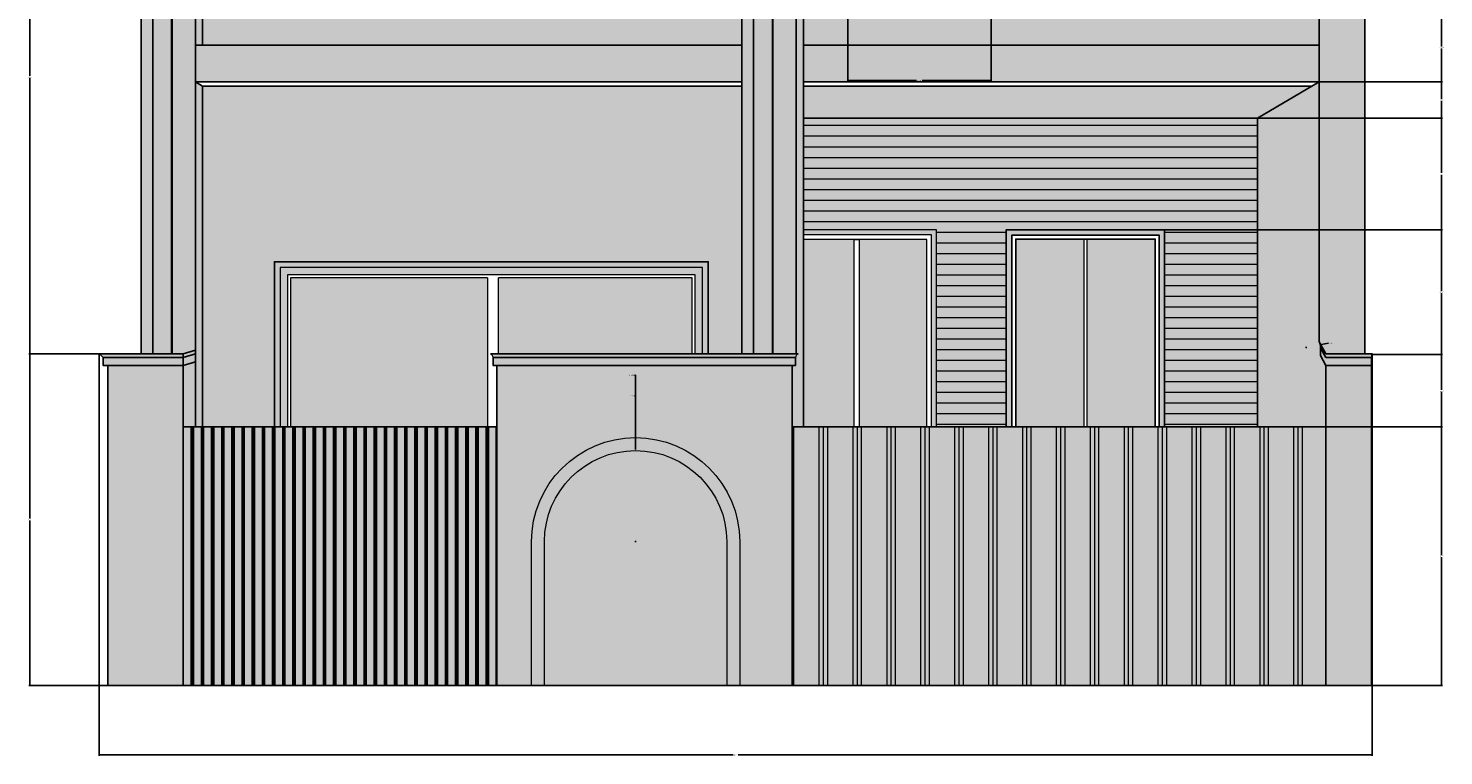
# Model space of a CAD drawing. Units: feet. Extents: x 2352 to 2983, y 950 to 1233.
# Tile 1 of 5: x 2352 to 2617, y 950 to 1086. Entities that reach past the tile are written whole.
import ezdxf

# ---------------------------------------------------------------- set-up
doc = ezdxf.new("R2010")
doc.units = ezdxf.units.FT
for name, color, linetype, lineweight in [('A-ANNO-DIMS', 2, 'Continuous', 18), ('A-DOOR', 3, 'Continuous', 18), ('A-ELEV', 7, 'Continuous', 25), ('A-ELEV-PATT', 252, 'Continuous', 13), ('A-GLAZ', 4, 'Continuous', 18)]:
    doc.layers.add(name, color=color, linetype=linetype, lineweight=lineweight)
doc.styles.get("Standard").update_dxf_attribs({"font": 'arial.ttf'})
doc.dimstyles.get("Standard").update_dxf_attribs({"dimtxt": 0.18, "dimasz": 0.18, "dimexe": 0.18, "dimexo": 0.0625, "dimgap": 0.09, "dimtad": 0, "dimtih": 1, "dimtoh": 1, "dimdec": 1, "dimzin": 0, "dimdsep": 46, "dimlunit": 3, "dimtxsty": 'Standard', "dimcen": 0.09, "dimadec": 0, "dimazin": 0, "dimtfac": 1, "dimtdec": 1, "dimtofl": 0, "dimtmove": 0, "dimatfit": 3, "dimfxl": 1, "dimtolj": 1, "dimtzin": 0, "dimarcsym": 0})

# ---------------------------------------------------------------- blocks, each defined once
blk = doc.blocks.new('*D4')
at = {"layer": 'A-ANNO-DIMS', "color": 0, "lineweight": -2, "transparency": 16777216}
for p, q in [((2505.64, 1088.95), (2505.64, 1076.24)), ((2532.49, 1088.95), (2532.49, 1076.24)), ((2505.82, 1076.42), (2518.53, 1076.42)), ((2532.31, 1076.42), (2519.59, 1076.42))]:
    blk.add_line(p, q, dxfattribs=at)
at = {"layer": 'A-ANNO-DIMS', "color": 0, "transparency": 16777216}
for points in [[(2505.82, 1076.45), (2505.82, 1076.39), (2505.64, 1076.42)], [(2532.31, 1076.45), (2532.31, 1076.39), (2532.49, 1076.42)]]:
    blk.add_solid(points, dxfattribs=at)
at = {"layer": 'Defpoints', "color": 0, "transparency": 16777216}
for p in [(2505.64, 1089.01), (2532.49, 1089.01), (2532.49, 1076.42)]:
    blk.add_point(p, dxfattribs=at)
at = {"layer": 'A-ANNO-DIMS', "color": 0, "transparency": 16777216, "insert": (2519.06, 1076.42), "char_height": 0.18, "attachment_point": 5}
blk.add_mtext('\\A1;27 TYP.', dxfattribs=at)
blk = doc.blocks.new('*D7')
at = {"layer": 'A-ANNO-DIMS', "color": 0, "lineweight": -2, "transparency": 16777216}
for p, q in [((2365.43, 1025.15), (2365.43, 949.88)), ((2603.87, 1024.98), (2603.87, 949.88)), ((2365.61, 950.06), (2484.19, 950.06)), ((2603.69, 950.06), (2485.12, 950.06))]:
    blk.add_line(p, q, dxfattribs=at)
at = {"layer": 'A-ANNO-DIMS', "color": 0, "transparency": 16777216}
for points in [[(2365.61, 950.09), (2365.61, 950.03), (2365.43, 950.06)], [(2603.69, 950.09), (2603.69, 950.03), (2603.87, 950.06)]]:
    blk.add_solid(points, dxfattribs=at)
at = {"layer": 'Defpoints', "color": 0, "transparency": 16777216}
for p in [(2365.43, 1025.21), (2603.87, 1025.04), (2603.87, 950.06)]:
    blk.add_point(p, dxfattribs=at)
at = {"layer": 'A-ANNO-DIMS', "color": 0, "transparency": 16777216, "insert": (2484.65, 950.06), "char_height": 0.18, "attachment_point": 5}
blk.add_mtext('\\A1;238.44', dxfattribs=at)
blk = doc.blocks.new('*D12')
at = {"layer": 'A-ANNO-DIMS', "color": 0, "lineweight": -2, "transparency": 16777216}
for p, q in [((2595.27, 1011.48), (2617.07, 1011.48)), ((2616.89, 1011.3), (2616.89, 987.43)), ((2616.89, 963.19), (2616.89, 987.07)), ((2595.27, 963.01), (2617.07, 963.01))]:
    blk.add_line(p, q, dxfattribs=at)
at = {"layer": 'A-ANNO-DIMS', "color": 0, "transparency": 16777216}
for points in [[(2616.86, 1011.3), (2616.92, 1011.3), (2616.89, 1011.48)], [(2616.86, 963.19), (2616.92, 963.19), (2616.89, 963.01)]]:
    blk.add_solid(points, dxfattribs=at)
at = {"layer": 'Defpoints', "color": 0, "transparency": 16777216}
for p in [(2595.21, 1011.48), (2616.89, 1011.48), (2595.21, 963.01)]:
    blk.add_point(p, dxfattribs=at)
at = {"layer": 'A-ANNO-DIMS', "color": 0, "transparency": 16777216, "insert": (2616.89, 987.25), "char_height": 0.18, "attachment_point": 5}
blk.add_mtext('\\A1;48.47', dxfattribs=at)
blk = doc.blocks.new('*D13')
at = {"layer": 'A-ANNO-DIMS', "color": 0, "lineweight": -2, "transparency": 16777216}
for p, q in [((2603.93, 1025.04), (2617.07, 1025.04)), ((2616.89, 1024.86), (2616.89, 1018.44)), ((2616.89, 1011.66), (2616.89, 1018.08)), ((2595.27, 1011.48), (2617.07, 1011.48))]:
    blk.add_line(p, q, dxfattribs=at)
at = {"layer": 'A-ANNO-DIMS', "color": 0, "transparency": 16777216}
for points in [[(2616.86, 1024.86), (2616.92, 1024.86), (2616.89, 1025.04)], [(2616.86, 1011.66), (2616.92, 1011.66), (2616.89, 1011.48)]]:
    blk.add_solid(points, dxfattribs=at)
at = {"layer": 'Defpoints', "color": 0, "transparency": 16777216}
for p in [(2603.87, 1025.04), (2616.89, 1025.04), (2595.21, 1011.48)]:
    blk.add_point(p, dxfattribs=at)
at = {"layer": 'A-ANNO-DIMS', "color": 0, "transparency": 16777216, "insert": (2616.89, 1018.26), "char_height": 0.18, "attachment_point": 5}
blk.add_mtext('\\A1;13.56', dxfattribs=at)
blk = doc.blocks.new('*D14')
at = {"layer": 'A-ANNO-DIMS', "color": 0, "lineweight": -2, "transparency": 16777216}
for p, q in [((2565.07, 1048.43), (2617.07, 1048.43)), ((2616.89, 1048.25), (2616.89, 1036.92)), ((2616.89, 1025.22), (2616.89, 1036.55)), ((2603.93, 1025.04), (2617.07, 1025.04))]:
    blk.add_line(p, q, dxfattribs=at)
at = {"layer": 'A-ANNO-DIMS', "color": 0, "transparency": 16777216}
for points in [[(2616.86, 1048.25), (2616.92, 1048.25), (2616.89, 1048.43)], [(2616.86, 1025.22), (2616.92, 1025.22), (2616.89, 1025.04)]]:
    blk.add_solid(points, dxfattribs=at)
at = {"layer": 'Defpoints', "color": 0, "transparency": 16777216}
for p in [(2565.01, 1048.43), (2616.89, 1048.43), (2603.87, 1025.04)]:
    blk.add_point(p, dxfattribs=at)
at = {"layer": 'A-ANNO-DIMS', "color": 0, "transparency": 16777216, "insert": (2616.89, 1036.74), "char_height": 0.18, "attachment_point": 5}
blk.add_mtext('\\A1;23.387', dxfattribs=at)
blk = doc.blocks.new('*D15')
at = {"layer": 'A-ANNO-DIMS', "color": 0, "lineweight": -2, "transparency": 16777216}
for p, q in [((2582.47, 1069.34), (2617.07, 1069.34)), ((2616.89, 1069.16), (2616.89, 1059.07)), ((2616.89, 1048.61), (2616.89, 1058.7)), ((2565.07, 1048.43), (2617.07, 1048.43))]:
    blk.add_line(p, q, dxfattribs=at)
at = {"layer": 'A-ANNO-DIMS', "color": 0, "transparency": 16777216}
for points in [[(2616.86, 1069.16), (2616.92, 1069.16), (2616.89, 1069.34)], [(2616.86, 1048.61), (2616.92, 1048.61), (2616.89, 1048.43)]]:
    blk.add_solid(points, dxfattribs=at)
at = {"layer": 'Defpoints', "color": 0, "transparency": 16777216}
for p in [(2582.41, 1069.34), (2616.89, 1069.34), (2565.01, 1048.43)]:
    blk.add_point(p, dxfattribs=at)
at = {"layer": 'A-ANNO-DIMS', "color": 0, "transparency": 16777216, "insert": (2616.89, 1058.88), "char_height": 0.18, "attachment_point": 5}
blk.add_mtext('\\A1;20.91', dxfattribs=at)
blk = doc.blocks.new('*D16')
at = {"layer": 'A-ANNO-DIMS', "color": 0, "lineweight": -2, "transparency": 16777216}
for p, q in [((2594.03, 1076.12), (2617.07, 1076.12)), ((2616.89, 1075.94), (2616.89, 1072.91)), ((2616.89, 1069.52), (2616.89, 1072.55)), ((2582.47, 1069.34), (2617.07, 1069.34))]:
    blk.add_line(p, q, dxfattribs=at)
at = {"layer": 'A-ANNO-DIMS', "color": 0, "transparency": 16777216}
for points in [[(2616.86, 1075.94), (2616.92, 1075.94), (2616.89, 1076.12)], [(2616.86, 1069.52), (2616.92, 1069.52), (2616.89, 1069.34)]]:
    blk.add_solid(points, dxfattribs=at)
at = {"layer": 'Defpoints', "color": 0, "transparency": 16777216}
for p in [(2593.97, 1076.12), (2616.89, 1076.12), (2582.41, 1069.34)]:
    blk.add_point(p, dxfattribs=at)
at = {"layer": 'A-ANNO-DIMS', "color": 0, "transparency": 16777216, "insert": (2616.89, 1072.73), "char_height": 0.18, "attachment_point": 5}
blk.add_mtext('\\A1;6.781', dxfattribs=at)
blk = doc.blocks.new('*D17')
at = {"layer": 'A-ANNO-DIMS', "color": 0, "lineweight": -2, "transparency": 16777216}
for p, q in [((2594.03, 1089.01), (2617.07, 1089.01)), ((2616.89, 1088.83), (2616.89, 1082.75)), ((2616.89, 1076.3), (2616.89, 1082.38)), ((2594.03, 1076.12), (2617.07, 1076.12))]:
    blk.add_line(p, q, dxfattribs=at)
at = {"layer": 'A-ANNO-DIMS', "color": 0, "transparency": 16777216}
for points in [[(2616.86, 1088.83), (2616.92, 1088.83), (2616.89, 1089.01)], [(2616.86, 1076.3), (2616.92, 1076.3), (2616.89, 1076.12)]]:
    blk.add_solid(points, dxfattribs=at)
at = {"layer": 'Defpoints', "color": 0, "transparency": 16777216}
for p in [(2593.97, 1089.01), (2616.89, 1089.01), (2593.97, 1076.12)]:
    blk.add_point(p, dxfattribs=at)
at = {"layer": 'A-ANNO-DIMS', "color": 0, "transparency": 16777216, "insert": (2616.89, 1082.57), "char_height": 0.18, "attachment_point": 5}
blk.add_mtext('\\A1;12.892', dxfattribs=at)
blk = doc.blocks.new('*D22')
at = {"layer": 'A-ANNO-DIMS', "color": 0, "lineweight": -2, "transparency": 16777216}
for p, q in [((2365.37, 1025.21), (2352.3, 1025.21)), ((2352.48, 1025.03), (2352.48, 994.3)), ((2352.48, 963.19), (2352.48, 993.93)), ((2367.01, 963.01), (2352.3, 963.01))]:
    blk.add_line(p, q, dxfattribs=at)
at = {"layer": 'A-ANNO-DIMS', "color": 0, "transparency": 16777216}
for points in [[(2352.45, 1025.03), (2352.51, 1025.03), (2352.48, 1025.21)], [(2352.45, 963.19), (2352.51, 963.19), (2352.48, 963.01)]]:
    blk.add_solid(points, dxfattribs=at)
at = {"layer": 'Defpoints', "color": 0, "transparency": 16777216}
for p in [(2352.48, 1025.21), (2365.43, 1025.21), (2367.07, 963.01)]:
    blk.add_point(p, dxfattribs=at)
at = {"layer": 'A-ANNO-DIMS', "color": 0, "transparency": 16777216, "insert": (2352.48, 994.11), "char_height": 0.18, "attachment_point": 5}
blk.add_mtext('\\A1;62.2', dxfattribs=at)
blk = doc.blocks.new('*D23')
at = {"layer": 'A-ANNO-DIMS', "color": 0, "lineweight": -2, "transparency": 16777216}
for p, q in [((2373.23, 1129.01), (2352.3, 1129.01)), ((2352.48, 1128.83), (2352.48, 1077.3)), ((2352.48, 1025.39), (2352.48, 1076.93)), ((2365.37, 1025.21), (2352.3, 1025.21))]:
    blk.add_line(p, q, dxfattribs=at)
at = {"layer": 'A-ANNO-DIMS', "color": 0, "transparency": 16777216}
for points in [[(2352.45, 1128.83), (2352.51, 1128.83), (2352.48, 1129.01)], [(2352.45, 1025.39), (2352.51, 1025.39), (2352.48, 1025.21)]]:
    blk.add_solid(points, dxfattribs=at)
at = {"layer": 'Defpoints', "color": 0, "transparency": 16777216}
for p in [(2352.48, 1129.01), (2373.3, 1129.01), (2365.43, 1025.21)]:
    blk.add_point(p, dxfattribs=at)
at = {"layer": 'A-ANNO-DIMS', "color": 0, "transparency": 16777216, "insert": (2352.48, 1077.11), "char_height": 0.18, "attachment_point": 5}
blk.add_mtext('\\A1;103.8', dxfattribs=at)
blk = doc.blocks.new('*D63')
at = {"layer": 'A-ANNO-DIMS', "color": 0, "lineweight": -2, "transparency": 16777216}
for p, q in [((2465.74, 1021.19), (2465.92, 1021.19)), ((2465.92, 1021.19), (2465.92, 1009.67)), ((2465.84, 989.99), (2466.02, 989.99)), ((2465.92, 989.9), (2465.92, 990.08))]:
    blk.add_line(p, q, dxfattribs=at)
at = {"layer": 'A-ANNO-DIMS', "color": 0, "transparency": 16777216}
blk.add_solid([(2465.95, 1009.67), (2465.89, 1009.67), (2465.92, 1009.49)], dxfattribs=at)
at = {"layer": 'Defpoints', "color": 0, "transparency": 16777216}
for p in [(2465.92, 1009.49), (2465.92, 989.99)]:
    blk.add_point(p, dxfattribs=at)
at = {"layer": 'A-ANNO-DIMS', "color": 0, "transparency": 16777216, "insert": (2465.2, 1021.19), "char_height": 0.18, "attachment_point": 5}
blk.add_mtext('\\A1;R19.497', dxfattribs=at)
blk = doc.blocks.new('*D64')
at = {"layer": 'A-ANNO-DIMS', "color": 0, "lineweight": -2, "transparency": 16777216}
for p, q in [((2465.74, 1017.31), (2465.92, 1017.31)), ((2465.92, 1017.31), (2465.92, 1007.24)), ((2465.84, 989.99), (2466.02, 989.99)), ((2465.92, 989.9), (2465.92, 990.08))]:
    blk.add_line(p, q, dxfattribs=at)
at = {"layer": 'A-ANNO-DIMS', "color": 0, "transparency": 16777216}
blk.add_solid([(2465.95, 1007.24), (2465.89, 1007.24), (2465.92, 1007.06)], dxfattribs=at)
at = {"layer": 'Defpoints', "color": 0, "transparency": 16777216}
for p in [(2465.92, 1007.06), (2465.92, 989.99)]:
    blk.add_point(p, dxfattribs=at)
at = {"layer": 'A-ANNO-DIMS', "color": 0, "transparency": 16777216, "insert": (2465.27, 1017.31), "char_height": 0.18, "attachment_point": 5}
blk.add_mtext('\\A1;R17.07', dxfattribs=at)
blk = doc.blocks.new('*D66')
at = {"layer": 'A-ANNO-DIMS', "color": 0, "lineweight": -2, "transparency": 16777216}
for p, q in [((2591.45, 1026.39), (2591.63, 1026.39)), ((2591.54, 1026.3), (2591.54, 1026.48)), ((2595.71, 1027.19), (2594.32, 1026.92))]:
    blk.add_line(p, q, dxfattribs=at)
at = {"layer": 'A-ANNO-DIMS', "color": 0, "transparency": 16777216}
blk.add_solid([(2594.31, 1026.95), (2594.33, 1026.89), (2594.14, 1026.89)], dxfattribs=at)
at = {"layer": 'Defpoints', "color": 0, "transparency": 16777216}
for p in [(2591.54, 1026.39), (2594.14, 1026.89)]:
    blk.add_point(p, dxfattribs=at)
at = {"layer": 'A-ANNO-DIMS', "color": 0, "transparency": 16777216, "insert": (2596.12, 1027.19), "char_height": 0.18, "attachment_point": 5}
blk.add_mtext('\\A1;R2.65', dxfattribs=at)

msp = doc.modelspace()

# ---------------------------------------------------------------- hatches: boundary and pattern name
at = {"layer": 'A-ELEV-PATT'}
h = msp.add_hatch(color=256, dxfattribs=at)
h.dxf.hatch_style = 1
h.paths.add_polyline_path([(2499.5465, 1215.0126), (2373.2965, 1215.0126), (2373.2965, 1209.0126), (2499.5465, 1209.0126)])
h.paths.add_polyline_path([(2502.6085, 1217.7513), (2403.3368, 1217.7513), (2373.2965, 1217.7513), (2373.2965, 1215.0126), (2499.5465, 1215.0126)])
h.paths.add_polyline_path([(2569.4416, 1219.8182), (2403.3368, 1219.8182), (2403.3368, 1217.7513), (2569.4416, 1217.7513)])
h.paths.add_polyline_path([(2593.9663, 1076.1207), (2582.4111, 1069.3398), (2582.4111, 1011.4831), (2595.2079, 1011.4831), (2595.2079, 1023.0126), (2594.1881, 1024.8551), (2594.1881, 1026.3357), (2594.1891, 1026.3338, 0.10932946), (2593.9663, 1027.4578)])
h.paths.add_polyline_path([(2602.5286, 1209.0126), (2593.9663, 1209.0126), (2593.9663, 1027.4578), (2595.2079, 1025.2146), (2602.5286, 1025.2146)])
h.paths.add_polyline_path([(2593.9663, 1083.0126), (2497.3422, 1083.0126), (2497.3422, 1076.1207), (2593.9663, 1076.1207)])
h.paths.add_polyline_path([(2485.8114, 1075.3288), (2384.8273, 1075.3288), (2384.8273, 1011.4831), (2398.2572, 1011.4831), (2398.2572, 1042.4514), (2479.5304, 1042.4514), (2479.5304, 1025.2146), (2485.8114, 1025.2146)])
h.paths.add_polyline_path([(2485.8114, 1083.0126), (2383.4779, 1083.0126), (2383.4779, 1076.1207), (2485.8114, 1076.1207)])
h.paths.add_polyline_path([(2495.9928, 1089.0126), (2491.6239, 1089.0126), (2491.6239, 1025.2146), (2495.9928, 1025.2146)])
h.paths.add_polyline_path([(2491.5297, 1089.0126), (2488.0105, 1089.0126), (2488.0105, 1025.2146), (2491.5297, 1025.2146)])
h.paths.add_polyline_path([(2379.0148, 1129.0147), (2375.4956, 1129.0147), (2375.4956, 1025.2146), (2379.0148, 1025.2146)])
h.paths.add_polyline_path([(2383.4779, 1129.0147), (2379.109, 1129.0147), (2379.109, 1025.2146), (2381.1604, 1025.2146), (2383.4779, 1025.8769)])
h.paths.add_polyline_path([(2389.4076, 1144.6653), (2389.4076, 1142.2389), (2384.8273, 1142.2389), (2384.8273, 1089.0126), (2397.2412, 1089.0126), (2397.2412, 1156.1636), (2471.8066, 1156.1636), (2471.8066, 1089.0126), (2485.8114, 1089.0126), (2485.8114, 1142.2389), (2480.0884, 1142.2389), (2480.0884, 1144.6653, 0.80625477)])
h.paths.add_polyline_path([(2389.4076, 1144.6653, -0.80625477), (2480.0884, 1144.6653, 1)])
h.paths.add_polyline_path([(2579.9743, 1185.4477), (2497.3422, 1185.4477), (2497.3422, 1147.0918), (2498.0576, 1146.9764), (2497.8725, 1144.5798, 0.11184527), (2497.3422, 1142.5724), (2497.3422, 1089.0126), (2505.6415, 1089.0126), (2505.6415, 1159.528, -1), (2532.4859, 1159.528), (2532.4859, 1089.0126), (2541.7346, 1089.0126), (2541.7346, 1159.528, -1), (2568.579, 1159.528), (2568.579, 1089.0126), (2579.9743, 1089.0126)])
h.paths.add_polyline_path([(2579.9743, 1191.2362), (2497.3422, 1191.2362), (2497.3422, 1185.4477), (2579.9743, 1185.4477)])
h.paths.add_polyline_path([(2381.1604, 1023.0126), (2367.0741, 1023.0126), (2367.0741, 963.0126), (2381.1604, 963.0126)])
h.paths.add_polyline_path([(2495.2282, 1011.4831), (2495.2282, 1023.0126), (2439.9479, 1023.0126), (2439.9479, 963.0126), (2446.428, 963.0126), (2446.428, 989.9926, -1), (2485.4222, 989.9926), (2485.4222, 963.0126), (2495.2282, 963.0126)])
h.paths.add_polyline_path([(2446.428, 989.9926), (2446.428, 963.0126), (2485.4222, 963.0126), (2485.4222, 989.9926, 1)], flags=17)
h.paths.add_polyline_path([(2603.7702, 1023.0126), (2595.2079, 1023.0126), (2595.2079, 1011.4831), (2595.2079, 963.0126), (2603.7702, 963.0126)])
h.paths.add_polyline_path([(2482.4531, 1147.0918), (2497.3422, 1147.0918), (2497.3422, 1185.4477), (2497.3422, 1194.3715), (2373.2965, 1194.3715), (2373.2965, 1147.0918), (2387.0428, 1147.0918, -0.95042953)])
h.paths.add_polyline_path([(2384.8273, 1142.2389), (2373.2965, 1142.2389), (2373.2965, 1129.0147), (2384.8273, 1129.0147)])
h.paths.add_polyline_path([(2495.9928, 1142.2389), (2488.0105, 1142.2389), (2488.0105, 1089.0126), (2491.5297, 1089.0126), (2495.9928, 1089.0126)])
h = msp.add_hatch(color=256, dxfattribs=at)
h.dxf.hatch_style = 1
h.paths.add_polyline_path([(2595.2079, 1011.4831), (2495.2282, 1011.4831), (2495.2282, 963.0126), (2595.2079, 963.0126)])
h.paths.add_polyline_path([(2579.9743, 1204.1231), (2569.4416, 1217.7513), (2502.6085, 1217.7513), (2499.5465, 1215.0126), (2499.5465, 1209.0126), (2497.3422, 1209.0126), (2497.3422, 1195.936), (2498.0772, 1195.936), (2498.0772, 1195.1775), (2497.8022, 1194.3715), (2497.3422, 1194.3715), (2497.3422, 1191.2362), (2579.9743, 1191.2362)])
h = msp.add_hatch(color=256, dxfattribs=at)
h.dxf.hatch_style = 1
h.paths.add_polyline_path([(2480.0884, 1144.6653), (2497.3422, 1144.6653), (2497.8725, 1144.5798), (2498.0576, 1146.9764), (2497.3422, 1147.0918), (2482.4531, 1147.0918, 0.95042953), (2387.0428, 1147.0918), (2373.2965, 1147.0918), (2371.8622, 1147.0918), (2372.5793, 1144.6653), (2389.4076, 1144.6653, -1)])
h.paths.add_polyline_path([(2389.4076, 1144.6653), (2372.5793, 1144.6653), (2373.2965, 1142.2389), (2389.4076, 1142.2389)])
h.paths.add_polyline_path([(2497.8725, 1144.5798), (2497.3422, 1144.6653), (2480.0884, 1144.6653), (2480.0884, 1142.2389), (2497.3422, 1142.2389, -0.12985075)])
h.paths.add_polyline_path([(2471.8066, 1156.1636), (2397.2412, 1156.1636), (2397.2412, 1089.0126), (2398.6146, 1089.0126), (2398.6146, 1154.7902), (2470.4332, 1154.7902), (2470.4332, 1089.0126), (2471.8066, 1089.0126)])
h.paths.add_polyline_path([(2470.4332, 1154.7902), (2398.6146, 1154.7902), (2398.6146, 1089.0126), (2400.114, 1089.0126), (2400.114, 1153.2908), (2468.9338, 1153.2908), (2468.9338, 1089.0126), (2470.4332, 1089.0126)], flags=17)
h.paths.add_polyline_path([(2495.8508, 1024.4932), (2439.2183, 1024.4932), (2439.2183, 1023.0126), (2495.8508, 1023.0126)])
h.paths.add_polyline_path([(2496.3417, 1025.2146), (2438.7275, 1025.2146, -0.22451739), (2439.2183, 1024.4932), (2495.8508, 1024.4932, -0.22451739)])
h.paths.add_polyline_path([(2381.1604, 1024.4932), (2366.1676, 1024.4932), (2366.1676, 1023.0126), (2381.1604, 1023.0126)])
h.paths.add_polyline_path([(2381.1604, 1025.2146), (2365.4325, 1025.2146, -0.12196493), (2366.1676, 1024.4932), (2381.1604, 1024.4932)])
h.paths.add_polyline_path([(2383.4779, 1025.1555), (2383.4779, 1025.8769), (2381.1604, 1025.2146), (2381.1604, 1024.4932)])
h.paths.add_polyline_path([(2383.4779, 1025.1555), (2381.1604, 1024.4932), (2381.1604, 1023.0126), (2383.4779, 1023.6749)])
h.paths.add_polyline_path([(2479.5304, 1042.4514), (2398.2572, 1042.4514), (2398.2572, 1011.4831), (2399.3703, 1011.4831), (2399.3703, 1041.3383), (2478.4174, 1041.3383), (2478.4174, 1025.2146), (2479.5304, 1025.2146)])
h.paths.add_polyline_path([(2478.4174, 1041.3383), (2399.3703, 1041.3383), (2399.3703, 1011.4831), (2400.6982, 1011.4831), (2400.6982, 1040.0104), (2477.0895, 1040.0104), (2477.0895, 1025.2146), (2478.4174, 1025.2146)], flags=17)
h.paths.add_polyline_path([(2565.0085, 1048.4289), (2535.3542, 1048.4289), (2535.3542, 1011.4831), (2536.3698, 1011.4831), (2536.3698, 1047.4133), (2563.993, 1047.4133), (2563.993, 1011.4831), (2565.0085, 1011.4831)])
h.paths.add_polyline_path([(2522.2926, 1048.4289), (2497.3422, 1048.4289), (2497.3422, 1047.4929), (2521.3566, 1047.4929), (2521.3566, 1011.4831), (2522.2926, 1011.4831)])
h.paths.add_polyline_path([(2603.9449, 1025.2146), (2603.7702, 1025.2146), (2595.2079, 1025.2146), (2593.9663, 1027.4578, -0.10932946), (2594.1891, 1026.3338), (2595.2079, 1024.4932), (2603.7702, 1024.4932, -0.10758073)])
h.paths.add_polyline_path([(2603.7702, 1024.4932), (2595.2079, 1024.4932), (2594.1891, 1026.3338, -0.00342101), (2594.1881, 1026.2975), (2594.1881, 1024.8551), (2595.2079, 1023.0126), (2603.7702, 1023.0126)])
h.paths.add_polyline_path([(2532.4859, 1159.528, 1), (2505.6415, 1159.528), (2505.6415, 1089.0126), (2505.9696, 1089.0126), (2505.9696, 1126.273), (2505.9696, 1159.528, -1), (2532.1578, 1159.528), (2532.1578, 1089.0126), (2532.4859, 1089.0126)])
h.paths.add_polyline_path([(2542.0627, 1159.528, -1), (2568.2509, 1159.528), (2568.2509, 1089.0126), (2568.579, 1089.0126), (2568.579, 1159.528, 1), (2541.7346, 1159.528), (2541.7346, 1089.0126), (2542.0627, 1089.0126)])
h.paths.add_polyline_path([(2522.687, 1127.7792), (2505.9696, 1127.7792), (2505.9696, 1126.273), (2511.9257, 1126.273), (2511.9257, 1089.0126), (2512.1488, 1089.0126), (2512.1488, 1126.273), (2521.1808, 1126.273), (2521.1808, 1089.0126), (2522.687, 1089.0126)], flags=17)
h.paths.add_polyline_path([(2439.9479, 1011.4831), (2381.1604, 1011.4831), (2381.1604, 963.0126), (2439.9479, 963.0126)])
h = msp.add_hatch(color=256, dxfattribs=at)
h.dxf.hatch_style = 1
h.paths.add_polyline_path([(2582.4111, 1069.3398), (2497.3422, 1069.3398), (2497.3422, 1048.4289), (2522.2926, 1048.4289), (2522.2926, 1011.4831), (2535.3542, 1011.4831), (2535.3542, 1048.4289), (2565.0085, 1048.4289), (2565.0085, 1011.4831), (2582.4111, 1011.4831)])
h.paths.add_polyline_path([(2568.2509, 1151.0596), (2542.0627, 1151.0596), (2542.0627, 1089.0126), (2568.2509, 1089.0126)])
h.paths.add_polyline_path([(2532.1578, 1151.0596), (2505.9696, 1151.0596), (2505.9696, 1127.7792), (2522.687, 1127.7792), (2522.687, 1089.0126), (2532.1578, 1089.0126)])
h.paths.add_polyline_path([(2505.9696, 1159.528), (2505.9696, 1151.0596), (2532.1578, 1151.0596), (2532.1578, 1159.528, 1)])
h.paths.add_polyline_path([(2568.2509, 1159.528, 1), (2542.0627, 1159.528), (2542.0627, 1151.0596), (2568.2509, 1151.0596)])
h = msp.add_hatch(color=256, dxfattribs=at)
h.dxf.hatch_style = 1
h.paths.add_polyline_path([(2438.1858, 1039.4184), (2401.2902, 1039.4184), (2401.2902, 1011.4831), (2438.1858, 1011.4831)])
h.paths.add_polyline_path([(2476.4975, 1039.4184), (2440.2408, 1039.4184), (2440.2408, 1025.2146), (2476.4975, 1025.2146)])
h.paths.add_polyline_path([(2563.252, 1046.6724), (2550.43, 1046.6724), (2550.43, 1011.4831), (2563.252, 1011.4831)])
h.paths.add_polyline_path([(2549.9328, 1046.6724), (2537.1107, 1046.6724), (2537.1107, 1011.4831), (2549.9328, 1011.4831)])
h.paths.add_polyline_path([(2520.4416, 1046.5779), (2507.7848, 1046.5779), (2507.7848, 1011.4831), (2520.4416, 1011.4831)])
h.paths.add_polyline_path([(2506.8593, 1046.5779), (2497.3422, 1046.5779), (2497.3422, 1011.4831), (2506.8593, 1011.4831)])
h.paths.add_polyline_path([(2521.1808, 1126.273), (2512.1488, 1126.273), (2512.1488, 1089.0126), (2521.1808, 1089.0126)])
h.paths.add_polyline_path([(2511.9257, 1126.273), (2505.9696, 1126.273), (2505.9696, 1089.0126), (2511.9257, 1089.0126)])
h.paths.add_polyline_path([(2466.1883, 1150.5453), (2435.4142, 1150.5453), (2435.4142, 1089.0126), (2466.1883, 1089.0126)])
h.paths.add_polyline_path([(2433.6336, 1150.5453), (2402.8595, 1150.5453), (2402.8595, 1089.0126), (2433.6336, 1089.0126)])
h = msp.add_hatch(dxfattribs=at)
h.set_pattern_fill('_USER', color=256, scale=2, pattern_type=0)
h.set_pattern_definition([(0, (0, 0), (0, 2), [])])
h.paths.add_polyline_path([(2532.1578, 1151.0596), (2505.9696, 1151.0596), (2505.9696, 1127.7792), (2522.687, 1127.7792), (2522.687, 1089.0126), (2532.1578, 1089.0126)])
h.paths.add_polyline_path([(2568.2509, 1151.0596), (2542.0627, 1151.0596), (2542.0627, 1089.0126), (2568.2509, 1089.0126)])
h.paths.add_polyline_path([(2582.4111, 1069.3398), (2497.3422, 1069.3398), (2497.3422, 1048.4289), (2522.2926, 1048.4289), (2522.2926, 1011.4831), (2535.3542, 1011.4831), (2535.3542, 1048.4289), (2565.0085, 1048.4289), (2565.0085, 1011.4831), (2582.4111, 1011.4831)])
h = msp.add_hatch(color=256, dxfattribs=at)
h.dxf.hatch_style = 1
h.paths.add_polyline_path([(2593.9663, 1089.0126), (2497.3422, 1089.0126), (2497.3422, 1083.0126), (2593.9663, 1083.0126)])
h.paths.add_polyline_path([(2485.8114, 1089.0126), (2384.8273, 1089.0126), (2384.8273, 1083.0126), (2485.8114, 1083.0126)])
h.paths.add_polyline_path([(2375.4956, 1129.0147), (2373.2965, 1129.0147), (2373.2965, 1025.2146), (2375.4956, 1025.2146)])
h.paths.add_polyline_path([(2384.8273, 1129.0147), (2383.4779, 1129.0147), (2383.4779, 1083.0126), (2384.8273, 1083.0126)])
h.paths.add_polyline_path([(2384.8273, 1075.3288), (2383.4779, 1076.1207), (2383.4779, 1025.8769), (2383.4779, 1011.4831), (2384.8273, 1011.4831)])
h.paths.add_polyline_path([(2488.0105, 1089.0126), (2485.8114, 1089.0126), (2485.8114, 1025.2146), (2488.0105, 1025.2146)])
h.paths.add_polyline_path([(2497.3422, 1089.0126), (2495.9928, 1089.0126), (2495.9928, 1025.2146), (2496.3417, 1025.2146, 0.22451739), (2495.8508, 1024.4932), (2495.8508, 1023.0126), (2495.2282, 1023.0126), (2495.2282, 1011.4831), (2497.3422, 1011.4831), (2497.3422, 1048.4289)])
h.paths.add_polyline_path([(2497.3422, 1142.2389), (2495.9928, 1142.2389), (2495.9928, 1089.0126), (2497.3422, 1089.0126)])
h.paths.add_polyline_path([(2488.0105, 1142.2389), (2485.8114, 1142.2389), (2485.8114, 1089.0126), (2488.0105, 1089.0126)])
h = msp.add_hatch(color=256, dxfattribs=at)
h.dxf.hatch_style = 1
h.paths.add_polyline_path([(2592.6169, 1075.3288), (2497.3422, 1075.3288), (2497.3422, 1069.3398), (2582.4111, 1069.3398)])
h = msp.add_hatch(color=256, dxfattribs=at)
h.dxf.hatch_style = 1
h.paths.add_polyline_path([(2383.4779, 1023.6749), (2381.1604, 1023.0126), (2381.1604, 1011.4831), (2383.4779, 1011.4831)])
h = msp.add_hatch(dxfattribs=at)
h.set_pattern_fill('PLAST', color=256, scale=0.3, angle=90)
h.paths.add_polyline_path([(2439.9479, 1011.4831), (2381.1604, 1011.4831), (2381.1604, 963.0126), (2439.9479, 963.0126)])
h = msp.add_hatch(dxfattribs=at)
h.set_pattern_fill('PLAST', color=256, angle=90)
h.paths.add_polyline_path([(2595.2079, 1011.4831), (2495.2282, 1011.4831), (2495.2282, 963.0126), (2595.2079, 963.0126)])
h = msp.add_hatch(color=256, dxfattribs=at)
h.dxf.hatch_style = 1
h.paths.add_polyline_path([(2446.428, 989.9926), (2446.428, 963.0126), (2448.8544, 963.0126), (2448.8544, 989.9926, -1), (2482.9957, 989.9926), (2482.9957, 963.0126), (2485.4222, 963.0126), (2485.4222, 989.9926, 1)])

# ---------------------------------------------------------------- linework, layer by layer
at = {"layer": 'A-DOOR'}
for points in [[(2497.3422, 1011.4831), (2522.2926, 1011.4831), (2522.2926, 1048.4289), (2497.3422, 1048.4289)], [(2497.3422, 1011.4831), (2522.2926, 1011.4831), (2522.2926, 1048.4289), (2497.3422, 1048.4289)], [(2506.8593, 1046.5779), (2507.7848, 1046.5779), (2507.7848, 1011.4831), (2506.8593, 1011.4831)], [(2506.8593, 1046.5779), (2507.7848, 1046.5779), (2507.7848, 1011.4831), (2506.8593, 1011.4831)], [(2549.9328, 1046.6724), (2550.43, 1046.6724), (2550.43, 1011.4831), (2549.9328, 1011.4831)], [(2549.9328, 1046.6724), (2550.43, 1046.6724), (2550.43, 1011.4831), (2549.9328, 1011.4831)]]:
    msp.add_lwpolyline(points, close=True, dxfattribs=at)
for points in [[(2521.3566, 1011.4831), (2521.3566, 1047.4929), (2497.3422, 1047.4929)], [(2521.3566, 1011.4831), (2521.3566, 1047.4929), (2497.3422, 1047.4929)], [(2520.4416, 1011.4831), (2520.4416, 1046.5779), (2497.3422, 1046.5779)], [(2520.4416, 1011.4831), (2520.4416, 1046.5779), (2497.3422, 1046.5779)]]:
    msp.add_lwpolyline(points, dxfattribs=at)
msp.add_lwpolyline([(2485.4222, 989.9926), (2485.4222, 963.0126), (2446.428, 963.0126), (2446.428, 989.9926, -1)], format="xyb", close=True, dxfattribs=at)
msp.add_lwpolyline([(2485.4222, 989.9926), (2485.4222, 963.0126), (2446.428, 963.0126), (2446.428, 989.9926, -1)], format="xyb", close=True, dxfattribs=at)
msp.add_lwpolyline([(2448.8544, 963.0126), (2448.8544, 989.9926, -1), (2482.9957, 989.9926), (2482.9957, 963.0126)], format="xyb", dxfattribs=at)
msp.add_arc((2496.8591, 1024.3349), 1.0206, 120.460852, 171.077099, dxfattribs=at)
msp.add_arc((2496.8591, 1024.3349), 1.0206, 120.460852, 171.077099, dxfattribs=at)
at = {"layer": 'A-ELEV'}
for p, q in [((2384.8273, 1083.0126), (2485.8114, 1083.0126)), ((2384.8273, 1083.0126), (2485.8114, 1083.0126)), ((2497.3422, 1083.0126), (2593.9663, 1083.0126)), ((2497.3422, 1083.0126), (2593.9663, 1083.0126)), ((2383.4779, 1076.1207), (2384.8273, 1075.3288)), ((2383.4779, 1076.1207), (2384.8273, 1075.3288)), ((2384.8273, 1075.3288), (2485.8114, 1075.3288)), ((2384.8273, 1075.3288), (2485.8114, 1075.3288)), ((2497.3422, 1075.3288), (2592.6169, 1075.3288)), ((2497.3422, 1075.3288), (2592.6169, 1075.3288)), ((2582.4111, 1069.3398), (2593.9663, 1076.1207)), ((2582.4111, 1069.3398), (2593.9663, 1076.1207)), ((2497.3422, 1069.3398), (2582.4111, 1069.3398)), ((2497.3422, 1069.3398), (2582.4111, 1069.3398)), ((2582.4111, 1069.3398), (2582.4111, 1011.4831)), ((2582.4111, 1069.3398), (2582.4111, 1011.4831)), ((2595.2079, 1025.2146), (2593.9663, 1027.4578)), ((2595.2079, 1025.2146), (2593.9663, 1027.4578)), ((2595.2079, 1024.4932), (2594.1881, 1026.3357)), ((2594.1881, 1024.8551), (2594.1881, 1026.3357)), ((2595.2079, 1024.4932), (2594.1881, 1026.3357)), ((2594.1881, 1024.8551), (2594.1881, 1026.3357)), ((2381.1604, 1025.2146), (2365.4325, 1025.2146)), ((2381.1604, 1025.2146), (2365.4325, 1025.2146)), ((2381.1604, 1025.2146), (2383.4779, 1025.8769)), ((2381.1604, 1025.2146), (2383.4779, 1025.8769)), ((2381.1604, 1024.4932), (2381.1604, 1025.2146)), ((2381.1604, 1024.4932), (2381.1604, 1025.2146)), ((2381.1604, 1024.4932), (2383.4779, 1025.1555)), ((2381.1604, 1024.4932), (2383.4779, 1025.1555)), ((2381.1604, 1023.0126), (2383.4779, 1023.6749)), ((2381.1604, 1023.0126), (2383.4779, 1023.6749)), ((2383.4779, 1011.4831), (2383.4779, 1025.8769)), ((2383.4779, 1011.4831), (2383.4779, 1025.8769)), ((2496.3417, 1025.2146), (2438.7275, 1025.2146)), ((2496.3417, 1025.2146), (2438.7275, 1025.2146)), ((2595.2079, 1023.0126), (2594.1881, 1024.8551)), ((2595.2079, 1023.0126), (2594.1881, 1024.8551)), ((2603.7702, 1025.2146), (2595.2079, 1025.2146)), ((2603.7702, 1025.2146), (2595.2079, 1025.2146)), ((2603.7702, 1025.2146), (2603.9449, 1025.2146)), ((2603.7702, 1025.2146), (2603.9449, 1025.2146)), ((2603.7702, 963.0126), (2603.7702, 1024.4932)), ((2603.7702, 963.0126), (2603.7702, 1024.4932)), ((2367.0741, 963.0126), (2367.0741, 1023.0126)), ((2367.0741, 963.0126), (2367.0741, 1023.0126)), ((2367.0741, 963.0126), (2367.0741, 1023.0126)), ((2367.0741, 963.0126), (2367.0741, 1023.0126)), ((2367.0741, 963.0126), (2603.7702, 963.0126)), ((2367.0741, 963.0126), (2603.7702, 963.0126))]:
    msp.add_line(p, q, dxfattribs=at)
for points in [[(2593.9663, 1027.4578), (2593.9663, 1209.0126)], [(2593.9663, 1027.4578), (2593.9663, 1209.0126)], [(2602.5286, 1209.0126), (2602.5286, 1025.2146), (2595.2079, 1025.2146)], [(2602.5286, 1209.0126), (2602.5286, 1025.2146), (2595.2079, 1025.2146)], [(2497.3422, 1142.5724), (2497.3422, 1011.4831)], [(2497.3422, 1142.5724), (2497.3422, 1011.4831)], [(2373.2965, 1025.2146), (2373.2965, 1142.2389)], [(2373.2965, 1025.2146), (2373.2965, 1142.2389)], [(2384.8273, 1142.2389), (2384.8273, 1083.0126)], [(2384.8273, 1142.2389), (2384.8273, 1083.0126)], [(2485.8114, 1025.2146), (2485.8114, 1142.2389)], [(2485.8114, 1025.2146), (2485.8114, 1142.2389)], [(2488.0105, 1025.2146), (2488.0105, 1142.2389)], [(2488.0105, 1025.2146), (2488.0105, 1142.2389)], [(2495.9928, 1142.2389), (2495.9928, 1025.2146)], [(2495.9928, 1142.2389), (2495.9928, 1025.2146)], [(2375.4956, 1025.2146), (2375.4956, 1129.0147)], [(2375.4956, 1025.2146), (2375.4956, 1129.0147)], [(2379.0148, 1129.0147), (2379.0148, 1025.2146), (2379.109, 1025.2146), (2379.109, 1129.0147)], [(2379.0148, 1129.0147), (2379.0148, 1025.2146), (2379.109, 1025.2146), (2379.109, 1129.0147)], [(2383.4779, 1129.0147), (2383.4779, 1025.8769)], [(2383.4779, 1129.0147), (2383.4779, 1025.8769)], [(2491.5297, 1089.0126), (2491.5297, 1025.2146), (2491.6239, 1025.2146), (2491.6239, 1089.0126)], [(2491.5297, 1089.0126), (2491.5297, 1025.2146), (2491.6239, 1025.2146), (2491.6239, 1089.0126)], [(2384.8273, 1075.3288), (2384.8273, 1011.4831), (2381.1604, 1011.4831)], [(2384.8273, 1075.3288), (2384.8273, 1011.4831), (2381.1604, 1011.4831)], [(2536.3698, 1011.4831), (2536.3698, 1047.4133), (2563.993, 1047.4133), (2563.993, 1011.4831)], [(2536.3698, 1011.4831), (2536.3698, 1047.4133), (2563.993, 1047.4133), (2563.993, 1011.4831)], [(2537.1107, 1011.4831), (2537.1107, 1046.6724), (2563.252, 1046.6724), (2563.252, 1011.4831)], [(2537.1107, 1011.4831), (2537.1107, 1046.6724), (2563.252, 1046.6724), (2563.252, 1011.4831)], [(2479.5304, 1025.2146), (2479.5304, 1042.4514), (2398.2572, 1042.4514), (2398.2572, 1011.4831)], [(2479.5304, 1025.2146), (2479.5304, 1042.4514), (2398.2572, 1042.4514), (2398.2572, 1011.4831)], [(2595.2079, 1024.4932), (2603.7702, 1024.4932), (2603.7702, 1023.0126), (2595.2079, 1023.0126)], [(2595.2079, 1024.4932), (2603.7702, 1024.4932), (2603.7702, 1023.0126), (2595.2079, 1023.0126)]]:
    msp.add_lwpolyline(points, dxfattribs=at)
for points in [[(2383.4779, 1083.0126), (2485.8114, 1083.0126), (2485.8114, 1076.1207), (2383.4779, 1076.1207)], [(2383.4779, 1083.0126), (2485.8114, 1083.0126), (2485.8114, 1076.1207), (2383.4779, 1076.1207)], [(2497.3422, 1083.0126), (2593.9663, 1083.0126), (2593.9663, 1076.1207), (2497.3422, 1076.1207)], [(2497.3422, 1083.0126), (2593.9663, 1083.0126), (2593.9663, 1076.1207), (2497.3422, 1076.1207)], [(2565.0085, 1011.4831), (2535.3542, 1011.4831), (2535.3542, 1048.4289), (2565.0085, 1048.4289)], [(2565.0085, 1011.4831), (2535.3542, 1011.4831), (2535.3542, 1048.4289), (2565.0085, 1048.4289)], [(2366.1676, 1024.4932), (2381.1604, 1024.4932), (2381.1604, 1023.0126), (2366.1676, 1023.0126)], [(2366.1676, 1024.4932), (2381.1604, 1024.4932), (2381.1604, 1023.0126), (2366.1676, 1023.0126)], [(2439.2183, 1024.4932), (2495.8508, 1024.4932), (2495.8508, 1023.0126), (2439.2183, 1023.0126)], [(2439.2183, 1024.4932), (2495.8508, 1024.4932), (2495.8508, 1023.0126), (2439.2183, 1023.0126)], [(2367.0741, 963.0126), (2381.1604, 963.0126), (2381.1604, 1023.0126), (2367.0741, 1023.0126)], [(2367.0741, 963.0126), (2381.1604, 963.0126), (2381.1604, 1023.0126), (2367.0741, 1023.0126)], [(2439.9479, 963.0126), (2495.2282, 963.0126), (2495.2282, 1023.0126), (2439.9479, 1023.0126)], [(2439.9479, 963.0126), (2495.2282, 963.0126), (2495.2282, 1023.0126), (2439.9479, 1023.0126)], [(2595.2079, 963.0126), (2603.7702, 963.0126), (2603.7702, 1023.0126), (2595.2079, 1023.0126)], [(2595.2079, 963.0126), (2603.7702, 963.0126), (2603.7702, 1023.0126), (2595.2079, 1023.0126)], [(2381.1604, 963.0126), (2439.9479, 963.0126), (2439.9479, 1011.4831), (2381.1604, 1011.4831)], [(2381.1604, 963.0126), (2439.9479, 963.0126), (2439.9479, 1011.4831), (2381.1604, 1011.4831)], [(2495.2282, 963.0126), (2595.2079, 963.0126), (2595.2079, 1011.4831), (2495.2282, 1011.4831)], [(2495.2282, 963.0126), (2595.2079, 963.0126), (2595.2079, 1011.4831), (2495.2282, 1011.4831)]]:
    msp.add_lwpolyline(points, close=True, dxfattribs=at)
for centre, radius, start, end in [((2591.5381, 1026.3923), 2.6517, 357.9519, 23.693279), ((2591.5381, 1026.3923), 2.6517, 357.9519, 23.693279), ((2364.3434, 1023.3696), 2.1425, 31.630035, 59.444961), ((2364.3434, 1023.3696), 2.1425, 31.630035, 59.444961), ((2605.5146, 1024.4527), 1.7448, 154.108905, 178.670129), ((2605.5146, 1024.4527), 1.7448, 154.108905, 178.670129)]:
    msp.add_arc(centre, radius, start, end, dxfattribs=at)
at = {"layer": 'A-GLAZ'}
for points in [[(2478.4174, 1025.2146), (2478.4174, 1041.3383), (2399.3703, 1041.3383), (2399.3703, 1011.4831)], [(2478.4174, 1025.2146), (2478.4174, 1041.3383), (2399.3703, 1041.3383), (2399.3703, 1011.4831)], [(2477.0895, 1025.2146), (2477.0895, 1040.0104), (2400.6982, 1040.0104), (2400.6982, 1011.4831)], [(2477.0895, 1025.2146), (2477.0895, 1040.0104), (2400.6982, 1040.0104), (2400.6982, 1011.4831)], [(2438.1858, 1039.4184), (2401.2902, 1039.4184), (2401.2902, 1011.4831)], [(2438.1858, 1039.4184), (2401.2902, 1039.4184), (2401.2902, 1011.4831)], [(2438.1858, 1039.4184), (2438.1858, 1011.4831)], [(2438.1858, 1039.4184), (2438.1858, 1011.4831)], [(2476.4975, 1025.2146), (2476.4975, 1039.4184), (2440.2408, 1039.4184)], [(2440.2408, 1025.2146), (2440.2408, 1039.4184)], [(2476.4975, 1025.2146), (2476.4975, 1039.4184), (2440.2408, 1039.4184)], [(2440.2408, 1025.2146), (2440.2408, 1039.4184)]]:
    msp.add_lwpolyline(points, dxfattribs=at)
msp.add_arc((2438.2101, 1024.3349), 1.0206, 8.922901, 59.539148, dxfattribs=at)
msp.add_arc((2438.2101, 1024.3349), 1.0206, 8.922901, 59.539148, dxfattribs=at)

# ---------------------------------------------------------------- dimensions: what is measured, and where the dimension line sits
at = {"layer": 'A-ANNO-DIMS'}
for base, p1, p2, override, picture, middle in [((2352.4825, 1129.0147), (2365.4325, 1025.2146), (2373.2965, 1129.0147), {"dimdec": 1, "dimlfac": 1, "dimrnd": 0, "dimzin": 0, "dimdsep": 46, "dimlunit": 2}, '*D23', (2352.4825, 1077.1147)), ((2616.8949, 1089.0126), (2593.9663, 1076.1207), (2593.9663, 1089.0126), {"dimdec": 3, "dimlfac": 1, "dimrnd": 0, "dimzin": 0, "dimdsep": 46, "dimlunit": 2}, '*D17', (2616.8949, 1082.5667)), ((2616.8949, 1076.1207), (2582.4111, 1069.3398), (2593.9663, 1076.1207), {"dimdec": 3, "dimlfac": 1, "dimrnd": 0, "dimzin": 0, "dimdsep": 46, "dimlunit": 2}, '*D16', (2616.8949, 1072.7303)), ((2616.8949, 1069.3398), (2565.0085, 1048.4289), (2582.4111, 1069.3398), {"dimdec": 2, "dimlfac": 1, "dimrnd": 0, "dimzin": 0, "dimdsep": 46, "dimlunit": 2}, '*D15', (2616.8949, 1058.8844)), ((2616.8949, 1048.4289), (2603.8723, 1025.0421), (2565.0085, 1048.4289), {"dimdec": 3, "dimlfac": 1, "dimrnd": 0, "dimzin": 0, "dimdsep": 46, "dimlunit": 2}, '*D14', (2616.8949, 1036.7355)), ((2352.4825, 1025.2146), (2367.0741, 963.0126), (2365.4325, 1025.2146), {"dimdec": 1, "dimlfac": 1, "dimrnd": 0, "dimzin": 0, "dimdsep": 46, "dimlunit": 2}, '*D22', (2352.4825, 994.1136)), ((2616.8949, 1025.0421), (2595.2079, 1011.4831), (2603.8723, 1025.0421), {"dimdec": 2, "dimlfac": 1, "dimrnd": 0, "dimzin": 0, "dimdsep": 46, "dimlunit": 2}, '*D13', (2616.8949, 1018.2626)), ((2616.8949, 1011.4831), (2595.2079, 963.0126), (2595.2079, 1011.4831), {"dimdec": 2, "dimlfac": 1, "dimrnd": 0, "dimzin": 0, "dimdsep": 46, "dimlunit": 2}, '*D12', (2616.8949, 987.2479))]:
    dim = msp.add_linear_dim(base=base, p1=p1, p2=p2, angle=90, dimstyle='Standard', override=override, dxfattribs=at)
    dim.commit()
    dim.dimension.update_dxf_attribs({"geometry": picture, "text_midpoint": middle})
dim = msp.add_linear_dim(base=(2532.4859, 1076.422), p1=(2505.6415, 1089.0126), p2=(2532.4859, 1089.0126), text='<> TYP.', dimstyle='Standard', override={"dimdec": 0, "dimrnd": 0, "dimzin": 0, "dimlunit": 2}, dxfattribs=at)
dim.commit()
dim.dimension.update_dxf_attribs({"geometry": '*D4', "text_midpoint": (2519.0637, 1076.422)})
for center, mpoint, override, picture, middle in [((2591.5381, 1026.3923), (2594.1427, 1026.8899), {"dimdec": 2, "dimlfac": 1, "dimrnd": 0, "dimzin": 0, "dimdsep": 46, "dimlunit": 2}, '*D66', (2595.7054, 1027.1885)), ((2465.9251, 989.9926), (2465.925, 1009.4897), {"dimdec": 3, "dimlfac": 1, "dimrnd": 0, "dimzin": 0, "dimdsep": 46, "dimlunit": 2}, '*D63', (2465.1952, 1021.188)), ((2465.9251, 989.9926), (2465.925, 1007.0633), {"dimdec": 2, "dimlfac": 1, "dimrnd": 0, "dimzin": 0, "dimdsep": 46, "dimlunit": 2}, '*D64', (2465.2651, 1017.3057))]:
    dim = msp.add_radius_dim(center=center, mpoint=mpoint, dimstyle='Standard', override=override, dxfattribs=at)
    dim.commit()
    dim.dimension.update_dxf_attribs({"geometry": picture, "text_midpoint": middle, "dimtype": 164})
dim = msp.add_linear_dim(base=(2603.8723, 950.0626), p1=(2365.4325, 1025.2146), p2=(2603.8723, 1025.0421), dimstyle='Standard', override={"dimdec": 2, "dimlfac": 1, "dimrnd": 0, "dimzin": 0, "dimdsep": 46, "dimlunit": 2}, dxfattribs=at)
dim.commit()
dim.dimension.update_dxf_attribs({"geometry": '*D7', "text_midpoint": (2484.6524, 950.0626)})

doc.saveas('drawing.dxf')
